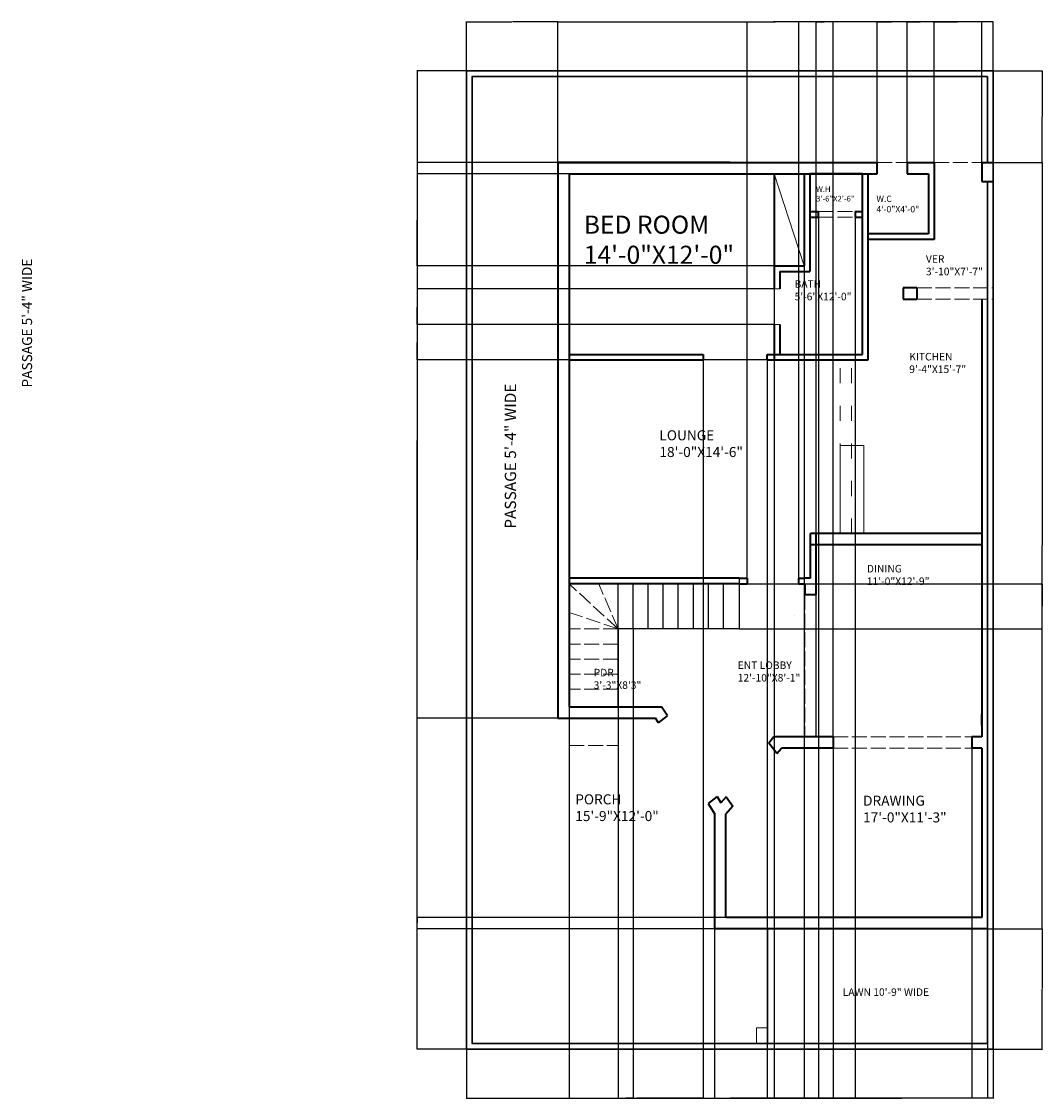
# Model space of a CAD drawing. Units: feet. Extents: x 1680 to 2494, y 1334 to 2193.
import ezdxf

# ---------------------------------------------------------------- set-up
doc = ezdxf.new("R2010")
doc.units = ezdxf.units.FT
doc.linetypes.add('ACAD_ISO02W100', pattern=[15, 12, -3])
doc.linetypes.add('ACAD_ISO03W100', pattern=[30, 12, -18])
for name, color, linetype, lineweight in [('A-ANNO-DIMS', 2, 'Continuous', 18), ('A-ANNO-REFR', 8, 'Continuous', 13), ('A-AREA-IDEN', 7, 'Continuous', 18), ('A-COLS', 7, 'Continuous', 35), ('A-FLOR-CASE', 8, 'Continuous', 18), ('A-FLOR-STRS', 7, 'Continuous', 25), ('A-FLOR-STRS-OVHD', 8, 'ACAD_ISO02W100', 18), ('A-SITE-OVHD', 8, 'ACAD_ISO02W100', 18), ('A-WALL', 7, 'Continuous', 35), ('A-WALL-OVHD', 8, 'ACAD_ISO02W100', 18), ('C-PROP', 7, 'Continuous', 30), ('L-SITE-EDGE', 3, 'Continuous', 18), ('S-BEAM-OVHD', 8, 'ACAD_ISO03W100', 18)]:
    doc.layers.add(name, color=color, linetype=linetype, lineweight=lineweight)
doc.styles.get("Standard").update_dxf_attribs({"font": 'arial.ttf'})
doc.dimstyles.get("Standard").update_dxf_attribs({"dimtxt": 0.18, "dimasz": 0.18, "dimexe": 0.18, "dimexo": 0.0625, "dimgap": 0.09, "dimtad": 0, "dimtih": 1, "dimtoh": 1, "dimdec": 4, "dimzin": 0, "dimdsep": 46, "dimtxsty": 'Standard', "dimcen": 0.09, "dimadec": 0, "dimazin": 0, "dimtfac": 1, "dimtdec": 4, "dimtofl": 0, "dimtmove": 0, "dimatfit": 3, "dimfxl": 1, "dimtolj": 1, "dimtzin": 0, "dimarcsym": 0})

# ---------------------------------------------------------------- blocks, each defined once
blk = doc.blocks.new('*D1')
at = {"layer": 'A-ANNO-DIMS', "color": 0, "lineweight": -2, "transparency": 16777216}
for p, q in [((2034.93, 1373.81), (2034.93, 1334.49)), ((2454.93, 1373.81), (2454.93, 1334.49)), ((2035.11, 1334.67), (2244.64, 1334.67)), ((2454.75, 1334.67), (2245.22, 1334.67))]:
    blk.add_line(p, q, dxfattribs=at)
at = {"layer": 'A-ANNO-DIMS', "color": 0, "transparency": 16777216}
for points in [[(2035.11, 1334.7), (2035.11, 1334.64), (2034.93, 1334.67)], [(2454.75, 1334.7), (2454.75, 1334.64), (2454.93, 1334.67)]]:
    blk.add_solid(points, dxfattribs=at)
at = {"layer": 'Defpoints', "color": 0, "transparency": 16777216}
for p in [(2034.93, 1373.87), (2454.93, 1373.87), (2454.93, 1334.67)]:
    blk.add_point(p, dxfattribs=at)
at = {"layer": 'A-ANNO-DIMS', "color": 0, "transparency": 16777216, "insert": (2244.93, 1334.67), "char_height": 0.18, "attachment_point": 5}
blk.add_mtext('\\A1;420', dxfattribs=at)
blk = doc.blocks.new('*D2')
at = {"layer": 'A-ANNO-DIMS', "color": 0, "lineweight": -2, "transparency": 16777216}
for p, q in [((2034.87, 2153.87), (1995.55, 2153.87)), ((1995.73, 2153.69), (1995.73, 1764.06)), ((1995.73, 1374.05), (1995.73, 1763.69)), ((2034.87, 1373.87), (1995.55, 1373.87))]:
    blk.add_line(p, q, dxfattribs=at)
at = {"layer": 'A-ANNO-DIMS', "color": 0, "transparency": 16777216}
for points in [[(1995.7, 2153.69), (1995.76, 2153.69), (1995.73, 2153.87)], [(1995.7, 1374.05), (1995.76, 1374.05), (1995.73, 1373.87)]]:
    blk.add_solid(points, dxfattribs=at)
at = {"layer": 'Defpoints', "color": 0, "transparency": 16777216}
for p in [(1995.73, 2153.87), (2034.93, 2153.87), (2034.93, 1373.87)]:
    blk.add_point(p, dxfattribs=at)
at = {"layer": 'A-ANNO-DIMS', "color": 0, "transparency": 16777216, "insert": (1995.73, 1763.87), "char_height": 0.18, "attachment_point": 5}
blk.add_mtext('\\A1;780', dxfattribs=at)
blk = doc.blocks.new('*D3')
at = {"layer": 'A-ANNO-DIMS', "color": 0, "lineweight": -2, "transparency": 16777216}
for p, q in [((2034.93, 2153.94), (2034.93, 2193.25)), ((2035.11, 2193.07), (2071.21, 2193.07)), ((2107.75, 2193.07), (2071.65, 2193.07)), ((2107.93, 2080.94), (2107.93, 2193.25))]:
    blk.add_line(p, q, dxfattribs=at)
at = {"layer": 'A-ANNO-DIMS', "color": 0, "transparency": 16777216}
for points in [[(2035.11, 2193.1), (2035.11, 2193.04), (2034.93, 2193.07)], [(2107.75, 2193.1), (2107.75, 2193.04), (2107.93, 2193.07)]]:
    blk.add_solid(points, dxfattribs=at)
at = {"layer": 'Defpoints', "color": 0, "transparency": 16777216}
for p in [(2107.93, 2193.07), (2034.93, 2153.87), (2107.93, 2080.87)]:
    blk.add_point(p, dxfattribs=at)
at = {"layer": 'A-ANNO-DIMS', "color": 0, "transparency": 16777216, "insert": (2071.43, 2193.07), "char_height": 0.18, "attachment_point": 5}
blk.add_mtext('\\A1;73', dxfattribs=at)
blk = doc.blocks.new('*D4')
at = {"layer": 'A-ANNO-DIMS', "color": 0, "lineweight": -2, "transparency": 16777216}
for p, q in [((2107.93, 2080.94), (2107.93, 2193.25)), ((2108.11, 2193.07), (2281.14, 2193.07)), ((2454.75, 2193.07), (2281.72, 2193.07)), ((2454.93, 2153.94), (2454.93, 2193.25))]:
    blk.add_line(p, q, dxfattribs=at)
at = {"layer": 'A-ANNO-DIMS', "color": 0, "transparency": 16777216}
for points in [[(2108.11, 2193.1), (2108.11, 2193.04), (2107.93, 2193.07)], [(2454.75, 2193.1), (2454.75, 2193.04), (2454.93, 2193.07)]]:
    blk.add_solid(points, dxfattribs=at)
at = {"layer": 'Defpoints', "color": 0, "transparency": 16777216}
for p in [(2454.93, 2193.07), (2454.93, 2153.87), (2107.93, 2080.87)]:
    blk.add_point(p, dxfattribs=at)
at = {"layer": 'A-ANNO-DIMS', "color": 0, "transparency": 16777216, "insert": (2281.43, 2193.07), "char_height": 0.18, "attachment_point": 5}
blk.add_mtext('\\A1;347', dxfattribs=at)
blk = doc.blocks.new('*D5')
at = {"layer": 'A-ANNO-DIMS', "color": 0, "lineweight": -2, "transparency": 16777216}
for p, q in [((2454.99, 2153.87), (2494.31, 2153.87)), ((2494.13, 2153.69), (2494.13, 2117.56)), ((2494.13, 2081.05), (2494.13, 2117.19)), ((2454.99, 2080.87), (2494.31, 2080.87))]:
    blk.add_line(p, q, dxfattribs=at)
at = {"layer": 'A-ANNO-DIMS', "color": 0, "transparency": 16777216}
for points in [[(2494.1, 2153.69), (2494.16, 2153.69), (2494.13, 2153.87)], [(2494.1, 2081.05), (2494.16, 2081.05), (2494.13, 2080.87)]]:
    blk.add_solid(points, dxfattribs=at)
at = {"layer": 'Defpoints', "color": 0, "transparency": 16777216}
for p in [(2454.93, 2153.87), (2454.93, 2080.87), (2494.13, 2080.87)]:
    blk.add_point(p, dxfattribs=at)
at = {"layer": 'A-ANNO-DIMS', "color": 0, "transparency": 16777216, "insert": (2494.13, 2117.37), "char_height": 0.18, "attachment_point": 5}
blk.add_mtext('\\A1;73', dxfattribs=at)
blk = doc.blocks.new('*D6')
at = {"layer": 'A-ANNO-DIMS', "color": 0, "lineweight": -2, "transparency": 16777216}
for p, q in [((2454.99, 2080.87), (2494.31, 2080.87)), ((2494.13, 2080.69), (2494.13, 1775.56)), ((2494.13, 1470.05), (2494.13, 1775.19)), ((2450.49, 1469.87), (2494.31, 1469.87))]:
    blk.add_line(p, q, dxfattribs=at)
at = {"layer": 'A-ANNO-DIMS', "color": 0, "transparency": 16777216}
for points in [[(2494.1, 2080.69), (2494.16, 2080.69), (2494.13, 2080.87)], [(2494.1, 1470.05), (2494.16, 1470.05), (2494.13, 1469.87)]]:
    blk.add_solid(points, dxfattribs=at)
at = {"layer": 'Defpoints', "color": 0, "transparency": 16777216}
for p in [(2454.93, 2080.87), (2450.43, 1469.87), (2494.13, 1469.87)]:
    blk.add_point(p, dxfattribs=at)
at = {"layer": 'A-ANNO-DIMS', "color": 0, "transparency": 16777216, "insert": (2494.13, 1775.37), "char_height": 0.18, "attachment_point": 5}
blk.add_mtext('\\A1;611', dxfattribs=at)
blk = doc.blocks.new('*D7')
at = {"layer": 'A-ANNO-DIMS', "color": 0, "lineweight": -2, "transparency": 16777216}
for p, q in [((2450.49, 1469.87), (2494.31, 1469.87)), ((2494.13, 1469.69), (2494.13, 1422.06)), ((2494.13, 1374.05), (2494.13, 1421.69)), ((2454.99, 1373.87), (2494.31, 1373.87))]:
    blk.add_line(p, q, dxfattribs=at)
at = {"layer": 'A-ANNO-DIMS', "color": 0, "transparency": 16777216}
for points in [[(2494.1, 1469.69), (2494.16, 1469.69), (2494.13, 1469.87)], [(2494.1, 1374.05), (2494.16, 1374.05), (2494.13, 1373.87)]]:
    blk.add_solid(points, dxfattribs=at)
at = {"layer": 'Defpoints', "color": 0, "transparency": 16777216}
for p in [(2450.43, 1469.87), (2454.93, 1373.87), (2494.13, 1373.87)]:
    blk.add_point(p, dxfattribs=at)
at = {"layer": 'A-ANNO-DIMS', "color": 0, "transparency": 16777216, "insert": (2494.13, 1421.87), "char_height": 0.18, "attachment_point": 5}
blk.add_mtext('\\A1;96', dxfattribs=at)
blk = doc.blocks.new('*D8')
at = {"layer": 'A-ANNO-DIMS', "color": 0, "lineweight": -2, "transparency": 16777216}
for p, q in [((2232.93, 1469.81), (2232.93, 1334.49)), ((2450.43, 1469.81), (2450.43, 1334.49)), ((2233.11, 1334.67), (2341.28, 1334.67)), ((2450.25, 1334.67), (2342.08, 1334.67))]:
    blk.add_line(p, q, dxfattribs=at)
at = {"layer": 'A-ANNO-DIMS', "color": 0, "transparency": 16777216}
for points in [[(2233.11, 1334.7), (2233.11, 1334.64), (2232.93, 1334.67)], [(2450.25, 1334.7), (2450.25, 1334.64), (2450.43, 1334.67)]]:
    blk.add_solid(points, dxfattribs=at)
at = {"layer": 'Defpoints', "color": 0, "transparency": 16777216}
for p in [(2232.93, 1469.87), (2450.43, 1469.87), (2450.43, 1334.67)]:
    blk.add_point(p, dxfattribs=at)
at = {"layer": 'A-ANNO-DIMS', "color": 0, "transparency": 16777216, "insert": (2341.68, 1334.67), "char_height": 0.18, "attachment_point": 5}
blk.add_mtext('\\A1;217.5', dxfattribs=at)
blk = doc.blocks.new('*D9')
at = {"layer": 'A-ANNO-DIMS', "color": 0, "lineweight": -2, "transparency": 16777216}
for p, q in [((2252.5, 1744.87), (2494.31, 1744.87)), ((2494.13, 1744.69), (2494.13, 1727.06)), ((2494.13, 1709.05), (2494.13, 1726.69)), ((2252.5, 1708.87), (2494.31, 1708.87))]:
    blk.add_line(p, q, dxfattribs=at)
at = {"layer": 'A-ANNO-DIMS', "color": 0, "transparency": 16777216}
for points in [[(2494.1, 1744.69), (2494.16, 1744.69), (2494.13, 1744.87)], [(2494.1, 1709.05), (2494.16, 1709.05), (2494.13, 1708.87)]]:
    blk.add_solid(points, dxfattribs=at)
at = {"layer": 'Defpoints', "color": 0, "transparency": 16777216}
for p in [(2252.44, 1744.87), (2494.13, 1744.87), (2252.44, 1708.87)]:
    blk.add_point(p, dxfattribs=at)
at = {"layer": 'A-ANNO-DIMS', "color": 0, "transparency": 16777216, "insert": (2494.13, 1726.87), "char_height": 0.18, "attachment_point": 5}
blk.add_mtext('\\A1;36', dxfattribs=at)
blk = doc.blocks.new('*D10')
at = {"layer": 'A-ANNO-DIMS', "color": 0, "lineweight": -2, "transparency": 16777216}
for p, q in [((2155.93, 1708.81), (2155.93, 1334.49)), ((2167.93, 1708.81), (2167.93, 1334.49)), ((2156.11, 1334.67), (2161.72, 1334.67)), ((2167.75, 1334.67), (2162.14, 1334.67))]:
    blk.add_line(p, q, dxfattribs=at)
at = {"layer": 'A-ANNO-DIMS', "color": 0, "transparency": 16777216}
for points in [[(2156.11, 1334.7), (2156.11, 1334.64), (2155.93, 1334.67)], [(2167.75, 1334.7), (2167.75, 1334.64), (2167.93, 1334.67)]]:
    blk.add_solid(points, dxfattribs=at)
at = {"layer": 'Defpoints', "color": 0, "transparency": 16777216}
for p in [(2155.93, 1708.87), (2167.93, 1708.87), (2167.93, 1334.67)]:
    blk.add_point(p, dxfattribs=at)
at = {"layer": 'A-ANNO-DIMS', "color": 0, "transparency": 16777216, "insert": (2161.93, 1334.67), "char_height": 0.18, "attachment_point": 5}
blk.add_mtext('\\A1;12', dxfattribs=at)
blk = doc.blocks.new('*D11')
at = {"layer": 'A-ANNO-DIMS', "color": 0, "lineweight": -2, "transparency": 16777216}
for p, q in [((2241.87, 1478.87), (1995.55, 1478.87)), ((1995.73, 1478.69), (1995.73, 1474.56)), ((2232.87, 1469.87), (1995.55, 1469.87)), ((1995.73, 1470.05), (1995.73, 1474.19))]:
    blk.add_line(p, q, dxfattribs=at)
at = {"layer": 'A-ANNO-DIMS', "color": 0, "transparency": 16777216}
for points in [[(1995.7, 1478.69), (1995.76, 1478.69), (1995.73, 1478.87)], [(1995.7, 1470.05), (1995.76, 1470.05), (1995.73, 1469.87)]]:
    blk.add_solid(points, dxfattribs=at)
at = {"layer": 'Defpoints', "color": 0, "transparency": 16777216}
for p in [(1995.73, 1478.87), (2241.93, 1478.87), (2232.93, 1469.87)]:
    blk.add_point(p, dxfattribs=at)
at = {"layer": 'A-ANNO-DIMS', "color": 0, "transparency": 16777216, "insert": (1995.73, 1474.37), "char_height": 0.18, "attachment_point": 5}
blk.add_mtext('\\A1;9', dxfattribs=at)
blk = doc.blocks.new('*D12')
at = {"layer": 'A-ANNO-DIMS', "color": 0, "lineweight": -2, "transparency": 16777216}
for p, q in [((2116.93, 1923.31), (2116.93, 1334.49)), ((2223.81, 1923.31), (2223.81, 1334.49)), ((2117.11, 1334.67), (2169.91, 1334.67)), ((2223.63, 1334.67), (2170.82, 1334.67))]:
    blk.add_line(p, q, dxfattribs=at)
at = {"layer": 'A-ANNO-DIMS', "color": 0, "transparency": 16777216}
for points in [[(2117.11, 1334.7), (2117.11, 1334.64), (2116.93, 1334.67)], [(2223.63, 1334.7), (2223.63, 1334.64), (2223.81, 1334.67)]]:
    blk.add_solid(points, dxfattribs=at)
at = {"layer": 'Defpoints', "color": 0, "transparency": 16777216}
for p in [(2116.93, 1923.37), (2223.81, 1923.37), (2223.81, 1334.67)]:
    blk.add_point(p, dxfattribs=at)
at = {"layer": 'A-ANNO-DIMS', "color": 0, "transparency": 16777216, "insert": (2170.37, 1334.67), "char_height": 0.18, "attachment_point": 5}
blk.add_mtext('\\A1;106.88', dxfattribs=at)
blk = doc.blocks.new('*D13')
at = {"layer": 'A-ANNO-DIMS', "color": 0, "lineweight": -2, "transparency": 16777216}
for p, q in [((2223.81, 1923.31), (2223.81, 1334.49)), ((2274.86, 1923.31), (2274.86, 1334.49)), ((2223.99, 1334.67), (2248.94, 1334.67)), ((2274.68, 1334.67), (2249.73, 1334.67))]:
    blk.add_line(p, q, dxfattribs=at)
at = {"layer": 'A-ANNO-DIMS', "color": 0, "transparency": 16777216}
for points in [[(2223.99, 1334.7), (2223.99, 1334.64), (2223.81, 1334.67)], [(2274.68, 1334.7), (2274.68, 1334.64), (2274.86, 1334.67)]]:
    blk.add_solid(points, dxfattribs=at)
at = {"layer": 'Defpoints', "color": 0, "transparency": 16777216}
for p in [(2223.81, 1923.37), (2274.86, 1923.37), (2274.86, 1334.67)]:
    blk.add_point(p, dxfattribs=at)
at = {"layer": 'A-ANNO-DIMS', "color": 0, "transparency": 16777216, "insert": (2249.33, 1334.67), "char_height": 0.18, "attachment_point": 5}
blk.add_mtext('\\A1;51.05', dxfattribs=at)
blk = doc.blocks.new('*D14')
at = {"layer": 'A-ANNO-DIMS', "color": 0, "lineweight": -2, "transparency": 16777216}
for p, q in [((2280.37, 1951.59), (1995.55, 1951.59)), ((1995.73, 1951.41), (1995.73, 1937.66)), ((1995.73, 1923.55), (1995.73, 1937.3)), ((2280.37, 1923.37), (1995.55, 1923.37))]:
    blk.add_line(p, q, dxfattribs=at)
at = {"layer": 'A-ANNO-DIMS', "color": 0, "transparency": 16777216}
for points in [[(1995.7, 1951.41), (1995.76, 1951.41), (1995.73, 1951.59)], [(1995.7, 1923.55), (1995.76, 1923.55), (1995.73, 1923.37)]]:
    blk.add_solid(points, dxfattribs=at)
at = {"layer": 'Defpoints', "color": 0, "transparency": 16777216}
for p in [(1995.73, 1951.59), (2280.43, 1951.59), (2280.43, 1923.37)]:
    blk.add_point(p, dxfattribs=at)
at = {"layer": 'A-ANNO-DIMS', "color": 0, "transparency": 16777216, "insert": (1995.73, 1937.48), "char_height": 0.18, "attachment_point": 5}
blk.add_mtext('\\A1;28.215', dxfattribs=at)
blk = doc.blocks.new('*D15')
at = {"layer": 'A-ANNO-DIMS', "color": 0, "lineweight": -2, "transparency": 16777216}
for p, q in [((2280.37, 1979.99), (1995.55, 1979.99)), ((1995.73, 1979.81), (1995.73, 1965.97)), ((1995.73, 1951.77), (1995.73, 1965.61)), ((2280.37, 1951.59), (1995.55, 1951.59))]:
    blk.add_line(p, q, dxfattribs=at)
at = {"layer": 'A-ANNO-DIMS', "color": 0, "transparency": 16777216}
for points in [[(1995.7, 1979.81), (1995.76, 1979.81), (1995.73, 1979.99)], [(1995.7, 1951.77), (1995.76, 1951.77), (1995.73, 1951.59)]]:
    blk.add_solid(points, dxfattribs=at)
at = {"layer": 'Defpoints', "color": 0, "transparency": 16777216}
for p in [(1995.73, 1979.99), (2280.43, 1979.99), (2280.43, 1951.59)]:
    blk.add_point(p, dxfattribs=at)
at = {"layer": 'A-ANNO-DIMS', "color": 0, "transparency": 16777216, "insert": (1995.73, 1965.79), "char_height": 0.18, "attachment_point": 5}
blk.add_mtext('\\A1;28.397', dxfattribs=at)
blk = doc.blocks.new('*D16')
at = {"layer": 'A-ANNO-DIMS', "color": 0, "lineweight": -2, "transparency": 16777216}
for p, q in [((2362.47, 2080.94), (2362.47, 2193.25)), ((2362.65, 2193.07), (2373.93, 2193.07)), ((2386.13, 2193.07), (2374.86, 2193.07)), ((2386.31, 2080.94), (2386.31, 2193.25))]:
    blk.add_line(p, q, dxfattribs=at)
at = {"layer": 'A-ANNO-DIMS', "color": 0, "transparency": 16777216}
for points in [[(2362.65, 2193.1), (2362.65, 2193.04), (2362.47, 2193.07)], [(2386.13, 2193.1), (2386.13, 2193.04), (2386.31, 2193.07)]]:
    blk.add_solid(points, dxfattribs=at)
at = {"layer": 'Defpoints', "color": 0, "transparency": 16777216}
for p in [(2386.31, 2193.07), (2362.47, 2080.87), (2386.31, 2080.87)]:
    blk.add_point(p, dxfattribs=at)
at = {"layer": 'A-ANNO-DIMS', "color": 0, "transparency": 16777216, "insert": (2374.39, 2193.07), "char_height": 0.18, "attachment_point": 5}
blk.add_mtext('\\A1;23.837', dxfattribs=at)
blk = doc.blocks.new('*D17')
at = {"layer": 'A-ANNO-DIMS', "color": 0, "lineweight": -2, "transparency": 16777216}
for p, q in [((2386.31, 2080.94), (2386.31, 2193.25)), ((2386.49, 2193.07), (2396.73, 2193.07)), ((2407.75, 2193.07), (2397.52, 2193.07)), ((2407.93, 2080.94), (2407.93, 2193.25))]:
    blk.add_line(p, q, dxfattribs=at)
at = {"layer": 'A-ANNO-DIMS', "color": 0, "transparency": 16777216}
for points in [[(2386.49, 2193.1), (2386.49, 2193.04), (2386.31, 2193.07)], [(2407.75, 2193.1), (2407.75, 2193.04), (2407.93, 2193.07)]]:
    blk.add_solid(points, dxfattribs=at)
at = {"layer": 'Defpoints', "color": 0, "transparency": 16777216}
for p in [(2407.93, 2193.07), (2386.31, 2080.87), (2407.93, 2080.87)]:
    blk.add_point(p, dxfattribs=at)
at = {"layer": 'A-ANNO-DIMS', "color": 0, "transparency": 16777216, "insert": (2397.12, 2193.07), "char_height": 0.18, "attachment_point": 5}
blk.add_mtext('\\A1;21.62', dxfattribs=at)
blk = doc.blocks.new('*D18')
at = {"layer": 'A-ANNO-DIMS', "color": 0, "lineweight": -2, "transparency": 16777216}
for p, q in [((2407.93, 2080.94), (2407.93, 2193.25)), ((2408.11, 2193.07), (2426.71, 2193.07)), ((2445.75, 2193.07), (2427.15, 2193.07)), ((2445.93, 2080.94), (2445.93, 2193.25))]:
    blk.add_line(p, q, dxfattribs=at)
at = {"layer": 'A-ANNO-DIMS', "color": 0, "transparency": 16777216}
for points in [[(2408.11, 2193.1), (2408.11, 2193.04), (2407.93, 2193.07)], [(2445.75, 2193.1), (2445.75, 2193.04), (2445.93, 2193.07)]]:
    blk.add_solid(points, dxfattribs=at)
at = {"layer": 'Defpoints', "color": 0, "transparency": 16777216}
for p in [(2445.93, 2193.07), (2407.93, 2080.87), (2445.93, 2080.87)]:
    blk.add_point(p, dxfattribs=at)
at = {"layer": 'A-ANNO-DIMS', "color": 0, "transparency": 16777216, "insert": (2426.93, 2193.07), "char_height": 0.18, "attachment_point": 5}
blk.add_mtext('\\A1;38', dxfattribs=at)
blk = doc.blocks.new('*D19')
at = {"layer": 'A-ANNO-DIMS', "color": 0, "lineweight": -2, "transparency": 16777216}
for p, q in [((2315.76, 2041.81), (2315.76, 1334.49)), ((2344.91, 2041.81), (2344.91, 1334.49)), ((2315.94, 1334.67), (2329.87, 1334.67)), ((2344.73, 1334.67), (2330.8, 1334.67))]:
    blk.add_line(p, q, dxfattribs=at)
at = {"layer": 'A-ANNO-DIMS', "color": 0, "transparency": 16777216}
for points in [[(2315.94, 1334.7), (2315.94, 1334.64), (2315.76, 1334.67)], [(2344.73, 1334.7), (2344.73, 1334.64), (2344.91, 1334.67)]]:
    blk.add_solid(points, dxfattribs=at)
at = {"layer": 'Defpoints', "color": 0, "transparency": 16777216}
for p in [(2315.76, 2041.87), (2344.91, 2041.87), (2344.91, 1334.67)]:
    blk.add_point(p, dxfattribs=at)
at = {"layer": 'A-ANNO-DIMS', "color": 0, "transparency": 16777216, "insert": (2330.33, 1334.67), "char_height": 0.18, "attachment_point": 5}
blk.add_mtext('\\A1;29.154', dxfattribs=at)
blk = doc.blocks.new('*D20')
at = {"layer": 'A-ANNO-DIMS', "color": 0, "lineweight": -2, "transparency": 16777216}
for p, q in [((2258.73, 1749.44), (2258.73, 2193.25)), ((2258.91, 2193.07), (2278.88, 2193.07)), ((2299.78, 2193.07), (2279.81, 2193.07)), ((2299.96, 1749.44), (2299.96, 2193.25))]:
    blk.add_line(p, q, dxfattribs=at)
at = {"layer": 'A-ANNO-DIMS', "color": 0, "transparency": 16777216}
for points in [[(2258.91, 2193.1), (2258.91, 2193.04), (2258.73, 2193.07)], [(2299.78, 2193.1), (2299.78, 2193.04), (2299.96, 2193.07)]]:
    blk.add_solid(points, dxfattribs=at)
at = {"layer": 'Defpoints', "color": 0, "transparency": 16777216}
for p in [(2299.96, 2193.07), (2258.73, 1749.37), (2299.96, 1749.37)]:
    blk.add_point(p, dxfattribs=at)
at = {"layer": 'A-ANNO-DIMS', "color": 0, "transparency": 16777216, "insert": (2279.34, 2193.07), "char_height": 0.18, "attachment_point": 5}
blk.add_mtext('\\A1;41.225', dxfattribs=at)
blk = doc.blocks.new('*D21')
at = {"layer": 'A-ANNO-DIMS', "color": 0, "lineweight": -2, "transparency": 16777216}
for p, q in [((2327.34, 1613.81), (2327.34, 1334.49)), ((2438.04, 1613.81), (2438.04, 1334.49)), ((2327.52, 1334.67), (2382.3, 1334.67)), ((2437.86, 1334.67), (2383.07, 1334.67))]:
    blk.add_line(p, q, dxfattribs=at)
at = {"layer": 'A-ANNO-DIMS', "color": 0, "transparency": 16777216}
for points in [[(2327.52, 1334.7), (2327.52, 1334.64), (2327.34, 1334.67)], [(2437.86, 1334.7), (2437.86, 1334.64), (2438.04, 1334.67)]]:
    blk.add_solid(points, dxfattribs=at)
at = {"layer": 'Defpoints', "color": 0, "transparency": 16777216}
for p in [(2327.34, 1613.87), (2438.04, 1613.87), (2438.04, 1334.67)]:
    blk.add_point(p, dxfattribs=at)
at = {"layer": 'A-ANNO-DIMS', "color": 0, "transparency": 16777216, "insert": (2382.69, 1334.67), "char_height": 0.18, "attachment_point": 5}
blk.add_mtext('\\A1;110.7', dxfattribs=at)
blk = doc.blocks.new('*D22')
at = {"layer": 'A-ANNO-DIMS', "color": 0, "lineweight": -2, "transparency": 16777216}
for p, q in [((2313.93, 1622.94), (2313.93, 2193.25)), ((2314.11, 2193.07), (2320.18, 2193.07)), ((2327.16, 2193.07), (2321.09, 2193.07)), ((2327.34, 1622.94), (2327.34, 2193.25))]:
    blk.add_line(p, q, dxfattribs=at)
at = {"layer": 'A-ANNO-DIMS', "color": 0, "transparency": 16777216}
for points in [[(2314.11, 2193.1), (2314.11, 2193.04), (2313.93, 2193.07)], [(2327.16, 2193.1), (2327.16, 2193.04), (2327.34, 2193.07)]]:
    blk.add_solid(points, dxfattribs=at)
at = {"layer": 'Defpoints', "color": 0, "transparency": 16777216}
for p in [(2327.34, 2193.07), (2313.93, 1622.87), (2327.34, 1622.87)]:
    blk.add_point(p, dxfattribs=at)
at = {"layer": 'A-ANNO-DIMS', "color": 0, "transparency": 16777216, "insert": (2320.63, 2193.07), "char_height": 0.18, "attachment_point": 5}
blk.add_mtext('\\A1;13.406', dxfattribs=at)
blk = doc.blocks.new('*D23')
at = {"layer": 'A-ANNO-DIMS', "color": 0, "lineweight": -2, "transparency": 16777216}
for p, q in [((2107.87, 2080.87), (1995.55, 2080.87)), ((1995.73, 2080.69), (1995.73, 1859.56)), ((1995.73, 1638.05), (1995.73, 1859.19)), ((2107.87, 1637.87), (1995.55, 1637.87))]:
    blk.add_line(p, q, dxfattribs=at)
at = {"layer": 'A-ANNO-DIMS', "color": 0, "transparency": 16777216}
for points in [[(1995.7, 2080.69), (1995.76, 2080.69), (1995.73, 2080.87)], [(1995.7, 1638.05), (1995.76, 1638.05), (1995.73, 1637.87)]]:
    blk.add_solid(points, dxfattribs=at)
at = {"layer": 'Defpoints', "color": 0, "transparency": 16777216}
for p in [(1995.73, 2080.87), (2107.93, 2080.87), (2107.93, 1637.87)]:
    blk.add_point(p, dxfattribs=at)
at = {"layer": 'A-ANNO-DIMS', "color": 0, "transparency": 16777216, "insert": (1995.73, 1859.37), "char_height": 0.18, "attachment_point": 5}
blk.add_mtext('\\A1;443', dxfattribs=at)
blk = doc.blocks.new('*D24')
at = {"layer": 'A-ANNO-DIMS', "color": 0, "lineweight": -2, "transparency": 16777216}
for p, q in [((2280.37, 2071.87), (1995.55, 2071.87)), ((1995.73, 2071.69), (1995.73, 2035.31)), ((1995.73, 1998.55), (1995.73, 2034.94)), ((2280.37, 1998.37), (1995.55, 1998.37))]:
    blk.add_line(p, q, dxfattribs=at)
at = {"layer": 'A-ANNO-DIMS', "color": 0, "transparency": 16777216}
for points in [[(1995.7, 2071.69), (1995.76, 2071.69), (1995.73, 2071.87)], [(1995.7, 1998.55), (1995.76, 1998.55), (1995.73, 1998.37)]]:
    blk.add_solid(points, dxfattribs=at)
at = {"layer": 'Defpoints', "color": 0, "transparency": 16777216}
for p in [(2280.43, 2071.87), (1995.73, 1998.37), (2280.43, 1998.37)]:
    blk.add_point(p, dxfattribs=at)
at = {"layer": 'A-ANNO-DIMS', "color": 0, "transparency": 16777216, "insert": (1995.73, 2035.12), "char_height": 0.18, "attachment_point": 5}
blk.add_mtext('\\A1;73.5', dxfattribs=at)
blk = doc.blocks.new('*D25')
at = {"layer": 'A-ANNO-DIMS', "color": 0, "lineweight": -2, "transparency": 16777216}
for p, q in [((2280.43, 2071.81), (2280.43, 1334.49)), ((2304.43, 2071.81), (2304.43, 1334.49)), ((2280.61, 1334.67), (2292.21, 1334.67)), ((2304.25, 1334.67), (2292.65, 1334.67))]:
    blk.add_line(p, q, dxfattribs=at)
at = {"layer": 'A-ANNO-DIMS', "color": 0, "transparency": 16777216}
for points in [[(2280.61, 1334.7), (2280.61, 1334.64), (2280.43, 1334.67)], [(2304.25, 1334.7), (2304.25, 1334.64), (2304.43, 1334.67)]]:
    blk.add_solid(points, dxfattribs=at)
at = {"layer": 'Defpoints', "color": 0, "transparency": 16777216}
for p in [(2280.43, 2071.87), (2304.43, 2071.87), (2304.43, 1334.67)]:
    blk.add_point(p, dxfattribs=at)
at = {"layer": 'A-ANNO-DIMS', "color": 0, "transparency": 16777216, "insert": (2292.43, 1334.67), "char_height": 0.18, "attachment_point": 5}
blk.add_mtext('\\A1;24', dxfattribs=at)

msp = doc.modelspace()

# ---------------------------------------------------------------- linework, layer by layer
at = {"layer": 'A-ANNO-REFR'}
msp.add_line((2296.5817, 1719.4648), (2296.5817, 1719.4648), dxfattribs=at)
msp.add_line((2296.5817, 1719.4648), (2296.5817, 1719.4648), dxfattribs=at)
at = {"layer": 'A-COLS'}
for p, q in [((2445.9308, 2080.874), (2445.9308, 2071.874)), ((2445.9308, 2080.874), (2454.9308, 2080.874)), ((2445.9308, 2071.874), (2445.9308, 2065.8007)), ((2445.9308, 2065.8007), (2454.9308, 2065.8007)), ((2394.0717, 1980.874), (2383.1979, 1980.874)), ((2383.1979, 1980.874), (2383.1979, 1971.874)), ((2394.0717, 1980.874), (2394.0717, 1971.874)), ((2383.1979, 1971.874), (2394.0717, 1971.874))]:
    msp.add_line(p, q, dxfattribs=at)
at = {"layer": 'A-FLOR-CASE'}
for p, q in [((2280.4308, 2071.874), (2304.4308, 1998.374)), ((2332.9308, 1855.2794), (2332.9308, 1784.874)), ((2351.8788, 1855.2794), (2332.9308, 1855.2794)), ((2351.8788, 1784.874), (2351.8788, 1855.2794))]:
    msp.add_line(p, q, dxfattribs=at)
at = {"layer": 'A-FLOR-STRS'}
for p, q in [((2155.9308, 1646.874), (2155.9308, 1744.874)), ((2167.9308, 1708.874), (2167.9308, 1744.874)), ((2179.9308, 1708.874), (2179.9308, 1744.874)), ((2191.9308, 1708.874), (2191.9308, 1744.874)), ((2191.9308, 1708.874), (2191.9308, 1744.874)), ((2203.9308, 1708.874), (2203.9308, 1744.874)), ((2215.9308, 1708.874), (2215.9308, 1744.874)), ((2227.9308, 1708.874), (2227.9308, 1744.874)), ((2239.9308, 1708.874), (2239.9308, 1744.874)), ((2252.439, 1749.374), (2252.439, 1708.874)), ((2252.439, 1708.874), (2155.9308, 1708.874))]:
    msp.add_line(p, q, dxfattribs=at)
at = {"layer": 'A-FLOR-STRS-OVHD'}
for p, q in [((2155.9308, 1708.874), (2116.9308, 1744.874)), ((2155.9308, 1708.874), (2116.9308, 1744.874)), ((2155.9308, 1708.874), (2140.5501, 1744.874)), ((2155.9308, 1708.874), (2116.9308, 1722.0134)), ((2155.9308, 1708.874), (2116.9308, 1708.874)), ((2155.9308, 1696.874), (2116.9308, 1696.874)), ((2155.9308, 1684.874), (2116.9308, 1684.874)), ((2155.9308, 1672.874), (2116.9308, 1672.874)), ((2155.9308, 1660.874), (2116.9308, 1660.874)), ((2116.9308, 1646.874), (2116.9308, 1615.9667)), ((2155.9308, 1646.874), (2155.9308, 1615.9667)), ((2116.9308, 1615.9667), (2155.9308, 1615.9667))]:
    msp.add_line(p, q, dxfattribs=at)
at = {"layer": 'A-SITE-OVHD'}
for p, q in [((2107.9308, 1637.874), (2039.4308, 1637.874)), ((2266.3292, 1390.825), (2275.3292, 1390.825))]:
    msp.add_line(p, q, dxfattribs=at)
at = {"layer": 'A-WALL'}
for p, q in [((2244.9308, 2080.874), (2107.9308, 2080.874)), ((2107.9308, 2080.874), (2362.4739, 2080.874)), ((2107.9308, 2080.874), (2107.9308, 1637.874)), ((2362.4739, 2071.874), (2362.4739, 2080.874)), ((2386.311, 2080.874), (2386.311, 2071.874)), ((2386.311, 2080.874), (2407.9308, 2080.874)), ((2407.9308, 2080.874), (2407.9308, 2019.374)), ((2116.9308, 2071.874), (2116.9308, 1646.874)), ((2116.9308, 2071.874), (2362.4739, 2071.874)), ((2116.9308, 2071.874), (2284.9308, 2071.874)), ((2116.9308, 2071.874), (2116.9308, 1927.874)), ((2280.4308, 2071.874), (2280.4308, 1979.9861)), ((2304.4308, 2071.874), (2304.4308, 2041.874)), ((2350.9308, 2071.874), (2308.9308, 2071.874)), ((2308.9308, 2071.874), (2308.9308, 2041.874)), ((2350.9308, 1927.874), (2350.9308, 2071.874)), ((2355.4308, 1923.374), (2355.4308, 2071.874)), ((2355.4308, 2071.874), (2362.4739, 2071.874)), ((2386.311, 2071.874), (2403.4308, 2071.874)), ((2386.311, 2071.874), (2403.4308, 2071.874)), ((2403.4308, 2071.874), (2403.4308, 2023.874)), ((2304.4308, 2041.874), (2304.4308, 1998.374)), ((2308.9308, 2041.874), (2315.7553, 2041.874)), ((2308.9308, 2041.874), (2308.9308, 1993.874)), ((2308.9308, 2037.374), (2315.7553, 2037.374)), ((2344.9093, 2041.874), (2350.9308, 2041.874)), ((2344.9093, 2037.374), (2350.9308, 2037.374)), ((2403.4308, 2023.874), (2355.4308, 2023.874)), ((2407.9308, 2019.374), (2355.4308, 2019.374)), ((2280.4308, 1998.374), (2304.4308, 1998.374)), ((2284.9308, 1993.874), (2284.9308, 1979.9861)), ((2284.9308, 1993.874), (2308.9308, 1993.874)), ((2445.9308, 1971.874), (2445.9308, 1784.874)), ((2280.4308, 1951.5891), (2280.4308, 1923.374)), ((2284.9308, 1951.5891), (2284.9308, 1927.874)), ((2116.9308, 1927.874), (2223.8066, 1927.874)), ((2274.859, 1927.874), (2284.9308, 1927.874)), ((2284.9308, 1927.874), (2350.9308, 1927.874)), ((2116.9308, 1923.374), (2223.8066, 1923.374)), ((2116.9308, 1923.374), (2223.8066, 1923.374)), ((2274.859, 1923.374), (2332.9308, 1923.374)), ((2274.859, 1923.374), (2284.9308, 1923.374)), ((2280.4308, 1923.374), (2355.4308, 1923.374)), ((2445.9308, 1805.1862), (2445.9308, 1652.1862)), ((2309.4308, 1749.374), (2309.4308, 1784.874)), ((2445.9308, 1784.874), (2309.4308, 1784.874)), ((2313.9308, 1736.2588), (2313.9308, 1784.874)), ((2445.9308, 1775.874), (2309.4308, 1775.874)), ((2445.9308, 1775.874), (2445.9308, 1631.874)), ((2445.9308, 1775.874), (2445.9308, 1622.874)), ((2252.439, 1749.374), (2116.9308, 1749.374)), ((2116.9308, 1744.874), (2116.9308, 1646.874)), ((2252.439, 1744.874), (2116.9308, 1744.874)), ((2252.439, 1749.374), (2258.732, 1749.374)), ((2252.439, 1744.874), (2258.732, 1744.874)), ((2258.732, 1749.374), (2258.732, 1744.874)), ((2299.9568, 1744.874), (2299.9568, 1749.374)), ((2299.9568, 1749.374), (2304.9308, 1749.374)), ((2299.9568, 1744.874), (2304.9308, 1744.874)), ((2309.4308, 1749.374), (2304.9308, 1749.374)), ((2304.9308, 1744.874), (2304.9308, 1736.2588)), ((2304.9308, 1736.2588), (2313.9308, 1736.2588)), ((2116.9308, 1646.874), (2155.9308, 1646.874)), ((2155.9308, 1646.874), (2171.6858, 1646.874)), ((2171.6858, 1646.874), (2186.2471, 1646.874)), ((2186.2471, 1646.874), (2190.4749, 1646.874)), ((2195.4006, 1639.5866), (2190.4749, 1646.874)), ((2445.9308, 1631.874), (2445.9308, 1640.874)), ((2107.9308, 1637.874), (2155.9308, 1637.874)), ((2155.9308, 1637.874), (2167.0655, 1637.874)), ((2167.0655, 1637.874), (2185.6951, 1637.874)), ((2188.2066, 1634.1583), (2185.6951, 1637.874)), ((2188.2066, 1634.1583), (2195.4006, 1639.5866)), ((2280.0242, 1622.874), (2276.0067, 1617.8321)), ((2282.5974, 1609.4808), (2276.0067, 1617.8321)), ((2286.2887, 1622.874), (2280.0242, 1622.874)), ((2304.9308, 1622.874), (2286.2887, 1622.874)), ((2327.337, 1622.874), (2304.9308, 1622.874)), ((2327.337, 1622.874), (2327.337, 1613.874)), ((2445.9308, 1622.874), (2438.0355, 1622.874)), ((2438.0355, 1622.874), (2438.0355, 1613.874)), ((2282.5974, 1609.4808), (2286.2887, 1613.874)), ((2327.337, 1613.874), (2286.2887, 1613.874)), ((2445.9308, 1613.874), (2438.0355, 1613.874)), ((2445.9308, 1613.874), (2445.9308, 1478.874)), ((2445.9308, 1582.874), (2445.9308, 1478.874)), ((2234.7914, 1575.2809), (2227.691, 1569.6416)), ((2234.7914, 1575.2809), (2237.8746, 1570.243)), ((2241.9898, 1575.1408), (2237.8746, 1570.243)), ((2241.9898, 1575.1408), (2247.3694, 1567.5529)), ((2241.9898, 1575.1408), (2247.3694, 1567.5529)), ((2227.691, 1569.6416), (2232.9308, 1561.0799)), ((2247.3694, 1567.5529), (2241.9308, 1561.0799)), ((2232.9308, 1469.874), (2232.9308, 1561.0799)), ((2241.9308, 1478.874), (2241.9308, 1561.0799)), ((2445.9308, 1478.874), (2241.9308, 1478.874)), ((2445.9308, 1478.874), (2241.9308, 1478.874)), ((2450.4308, 1469.874), (2232.9308, 1469.874))]:
    msp.add_line(p, q, dxfattribs=at)
for points in [[(2315.7553, 2037.374), (2315.7553, 2041.874)], [(2344.9093, 2041.874), (2344.9093, 2037.374)], [(2223.8066, 1927.874), (2223.8066, 1923.374)], [(2274.859, 1923.374), (2274.859, 1927.874)]]:
    msp.add_lwpolyline(points, dxfattribs=at)
at = {"layer": 'A-WALL-OVHD'}
for p, q in [((2362.4739, 2080.874), (2386.311, 2080.874)), ((2407.9308, 2080.874), (2445.9308, 2080.874)), ((2315.7553, 2041.874), (2344.9093, 2041.874)), ((2315.7553, 2037.374), (2344.9093, 2037.374)), ((2394.0717, 1980.874), (2454.9308, 1980.874)), ((2394.0717, 1971.874), (2454.9308, 1971.874)), ((2304.9308, 1736.2588), (2304.9308, 1622.874)), ((2313.9308, 1736.2588), (2313.9308, 1622.874)), ((2327.337, 1622.874), (2438.0355, 1622.874)), ((2327.337, 1613.874), (2438.0355, 1613.874))]:
    msp.add_line(p, q, dxfattribs=at)
for points in [[(2280.4308, 1979.9861), (2284.9308, 1979.9861)], [(2284.9308, 1951.5891), (2280.4308, 1951.5891)]]:
    msp.add_lwpolyline(points, dxfattribs=at)
at = {"layer": 'C-PROP'}
msp.add_lwpolyline([(2454.9308, 2153.874), (2454.9308, 1373.874), (2034.9308, 1373.874), (2034.9308, 2153.874)], close=True, dxfattribs=at)
msp.add_lwpolyline([(2450.4308, 2065.8007), (2450.4308, 1378.374), (2039.4308, 1378.374), (2039.4308, 2149.374), (2450.4308, 2149.374), (2450.4308, 2080.874)], dxfattribs=at)
at = {"layer": 'L-SITE-EDGE'}
for p, q in [((2275.3292, 1399.2325), (2275.3292, 1469.874)), ((2275.3292, 1399.2325), (2275.3292, 1378.374)), ((2266.3292, 1390.825), (2266.3292, 1378.374))]:
    msp.add_line(p, q, dxfattribs=at)
at = {"layer": 'S-BEAM-OVHD'}
for p, q in [((2332.9308, 1784.874), (2332.9308, 1923.374)), ((2341.9308, 1784.874), (2341.9308, 1923.374))]:
    msp.add_line(p, q, dxfattribs=at)

# ---------------------------------------------------------------- texts
at = {"layer": 'A-AREA-IDEN', "attachment_point": 1}
for s, insert, char_height in [('W.H\\P3\'-6"X2\'-6"', (2313.8218, 2061.7566), 4.5), ('W.C\\P4\'-0"X4\'-0"', (2361.9401, 2054.4535), 5), ('BED ROOM \\P14\'-0"X12\'-0"', (2128.5676, 2038.4782), 14.4), ('VER\\P3\'-10"X7\'-7"', (2401.4196, 2006.9285), 6), ('BATH\\P5\'-6"X12\'-0"', (2296.6571, 1986.9623), 6), ('KITCHEN\\P9\'-4"X15\'-7"', (2388.0985, 1928.9946), 6), ('LOUNGE\\P18\'-0"X14\'-6"', (2188.8657, 1867.3243), 8), ('DINING\\P11\'-0"X12\'-9"', (2354.3071, 1759.9408), 6), ('PDR\\P3\'-3"X8\'3"', (2136.4308, 1677.1073), 6), ('ENT LOBBY\\P12\'-10"X8\'-1"', (2251.3196, 1682.9838), 6), ('PORCH\\P15\'-9"X12\'-0"', (2121.7513, 1577.0304), 8), ('DRAWING\\P17\'-0"X11\'-3"', (2351.3022, 1575.9485), 8), ('LAWN 10\'-9" WIDE', (2335.0604, 1422.3137), 6)]:
    msp.add_mtext_dynamic_manual_height_columns(s, width=153.116714, gutter_width=12.5, heights=[0], dxfattribs=dict(at, insert=insert, char_height=char_height))
at = {"layer": 'A-AREA-IDEN', "attachment_point": 1, "rotation": 90}
for s, insert, char_height in [('PASSAGE 5\'-4" WIDE', (1680.6011, 1901.3994), 8), ('PASSAGE 5\'-4" WIDE ', (2065.548, 1788.8303), 9)]:
    msp.add_mtext_dynamic_manual_height_columns(s, width=153.116714, gutter_width=12.5, heights=[0], dxfattribs=dict(at, insert=insert, char_height=char_height))

# ---------------------------------------------------------------- dimensions: what is measured, and where the dimension line sits
at = {"layer": 'A-ANNO-DIMS'}
for base, p1, p2, override, picture, middle in [((2107.9308, 2193.074), (2034.9308, 2153.874), (2107.9308, 2080.874), {"dimdec": 0, "dimlfac": 1, "dimrnd": 0, "dimzin": 0, "dimdsep": 46, "dimlunit": 2}, '*D3', (2071.4308, 2193.074)), ((2454.9308, 2193.074), (2107.9308, 2080.874), (2454.9308, 2153.874), {"dimdec": 0, "dimlfac": 1, "dimrnd": 0, "dimzin": 0, "dimdsep": 46, "dimlunit": 2}, '*D4', (2281.4308, 2193.074)), ((2299.9568, 2193.074), (2258.732, 1749.374), (2299.9568, 1749.374), {"dimdec": 3, "dimlfac": 1, "dimrnd": 0, "dimzin": 0, "dimdsep": 46, "dimlunit": 2}, '*D20', (2279.3444, 2193.074)), ((2327.337, 2193.074), (2313.9308, 1622.874), (2327.337, 1622.874), {"dimdec": 3, "dimlfac": 1, "dimrnd": 0, "dimzin": 0, "dimdsep": 46, "dimlunit": 2}, '*D22', (2320.6339, 2193.074)), ((2386.311, 2193.074), (2362.4739, 2080.874), (2386.311, 2080.874), {"dimdec": 3, "dimlfac": 1, "dimrnd": 0, "dimzin": 0, "dimdsep": 46, "dimlunit": 2}, '*D16', (2374.3924, 2193.074)), ((2407.9308, 2193.074), (2386.311, 2080.874), (2407.9308, 2080.874), {"dimdec": 2, "dimlfac": 1, "dimrnd": 0, "dimzin": 0, "dimdsep": 46, "dimlunit": 2}, '*D17', (2397.1209, 2193.074)), ((2445.9308, 2193.074), (2407.9308, 2080.874), (2445.9308, 2080.874), {"dimdec": 0, "dimlfac": 1, "dimrnd": 0, "dimzin": 0, "dimdsep": 46, "dimlunit": 2}, '*D18', (2426.9308, 2193.074)), ((2304.4308, 1334.674), (2280.4308, 2071.874), (2304.4308, 2071.874), {"dimdec": 0, "dimlfac": 1, "dimrnd": 0, "dimzin": 0, "dimdsep": 46, "dimlunit": 2}, '*D25', (2292.4308, 1334.674)), ((2344.9093, 1334.674), (2315.7553, 2041.874), (2344.9093, 2041.874), {"dimdec": 3, "dimlfac": 1, "dimrnd": 0, "dimzin": 0, "dimdsep": 46, "dimlunit": 2}, '*D19', (2330.3323, 1334.674)), ((2223.8066, 1334.674), (2116.9308, 1923.374), (2223.8066, 1923.374), {"dimdec": 2, "dimlfac": 1, "dimrnd": 0, "dimzin": 0, "dimdsep": 46, "dimlunit": 2}, '*D12', (2170.3687, 1334.674)), ((2274.859, 1334.674), (2223.8066, 1923.374), (2274.859, 1923.374), {"dimdec": 2, "dimlfac": 1, "dimrnd": 0, "dimzin": 0, "dimdsep": 46, "dimlunit": 2}, '*D13', (2249.3328, 1334.674)), ((2167.9308, 1334.674), (2155.9308, 1708.874), (2167.9308, 1708.874), {"dimdec": 0, "dimlfac": 1, "dimrnd": 0, "dimzin": 0, "dimdsep": 46, "dimlunit": 2}, '*D10', (2161.9308, 1334.674)), ((2438.0355, 1334.674), (2327.337, 1613.874), (2438.0355, 1613.874), {"dimdec": 1, "dimlfac": 1, "dimrnd": 0, "dimzin": 0, "dimdsep": 46, "dimlunit": 2}, '*D21', (2382.6863, 1334.674)), ((2450.4308, 1334.674), (2232.9308, 1469.874), (2450.4308, 1469.874), {"dimdec": 1, "dimlfac": 1, "dimrnd": 0, "dimzin": 0, "dimdsep": 46, "dimlunit": 2}, '*D8', (2341.6808, 1334.674)), ((2454.9308, 1334.674), (2034.9308, 1373.874), (2454.9308, 1373.874), {"dimdec": 0, "dimlfac": 1, "dimrnd": 0, "dimzin": 0, "dimdsep": 46, "dimlunit": 2}, '*D1', (2244.9308, 1334.674))]:
    dim = msp.add_linear_dim(base=base, p1=p1, p2=p2, dimstyle='Standard', override=override, dxfattribs=at)
    dim.commit()
    dim.dimension.update_dxf_attribs({"geometry": picture, "text_midpoint": middle})
for base, p1, p2, override, picture, middle in [((1995.7308, 2153.874), (2034.9308, 1373.874), (2034.9308, 2153.874), {"dimdec": 0, "dimlfac": 1, "dimrnd": 0, "dimzin": 0, "dimdsep": 46, "dimlunit": 2}, '*D2', (1995.7308, 1763.874)), ((2494.1308, 2080.874), (2454.9308, 2153.874), (2454.9308, 2080.874), {"dimdec": 0, "dimlfac": 1, "dimrnd": 0, "dimzin": 0, "dimdsep": 46, "dimlunit": 2}, '*D5', (2494.1308, 2117.374)), ((1995.7308, 2080.874), (2107.9308, 1637.874), (2107.9308, 2080.874), {"dimdec": 0, "dimlfac": 1, "dimrnd": 0, "dimzin": 0, "dimdsep": 46, "dimlunit": 2}, '*D23', (1995.7308, 1859.374)), ((2494.1308, 1469.874), (2454.9308, 2080.874), (2450.4308, 1469.874), {"dimdec": 0, "dimlfac": 1, "dimrnd": 0, "dimzin": 0, "dimdsep": 46, "dimlunit": 2}, '*D6', (2494.1308, 1775.374)), ((1995.7308, 1998.374), (2280.4308, 2071.874), (2280.4308, 1998.374), {"dimdec": 1, "dimlfac": 1, "dimrnd": 0, "dimzin": 0, "dimdsep": 46, "dimlunit": 2}, '*D24', (1995.7308, 2035.124)), ((1995.7308, 1979.9861), (2280.4308, 1951.5891), (2280.4308, 1979.9861), {"dimdec": 3, "dimlfac": 1, "dimrnd": 0, "dimzin": 0, "dimdsep": 46, "dimlunit": 2}, '*D15', (1995.7308, 1965.7876)), ((1995.7308, 1951.5891), (2280.4308, 1923.374), (2280.4308, 1951.5891), {"dimdec": 3, "dimlfac": 1, "dimrnd": 0, "dimzin": 0, "dimdsep": 46, "dimlunit": 2}, '*D14', (1995.7308, 1937.4815)), ((2494.1308, 1744.874), (2252.439, 1708.874), (2252.439, 1744.874), {"dimdec": 0, "dimlfac": 1, "dimrnd": 0, "dimzin": 0, "dimdsep": 46, "dimlunit": 2}, '*D9', (2494.1308, 1726.874)), ((1995.7308, 1478.874), (2232.9308, 1469.874), (2241.9308, 1478.874), {"dimdec": 0, "dimlfac": 1, "dimrnd": 0, "dimzin": 0, "dimdsep": 46, "dimlunit": 2}, '*D11', (1995.7308, 1474.374)), ((2494.1308, 1373.874), (2450.4308, 1469.874), (2454.9308, 1373.874), {"dimdec": 0, "dimlfac": 1, "dimrnd": 0, "dimzin": 0, "dimdsep": 46, "dimlunit": 2}, '*D7', (2494.1308, 1421.874))]:
    dim = msp.add_linear_dim(base=base, p1=p1, p2=p2, angle=90, dimstyle='Standard', override=override, dxfattribs=at)
    dim.commit()
    dim.dimension.update_dxf_attribs({"geometry": picture, "text_midpoint": middle})

doc.saveas('drawing.dxf')
